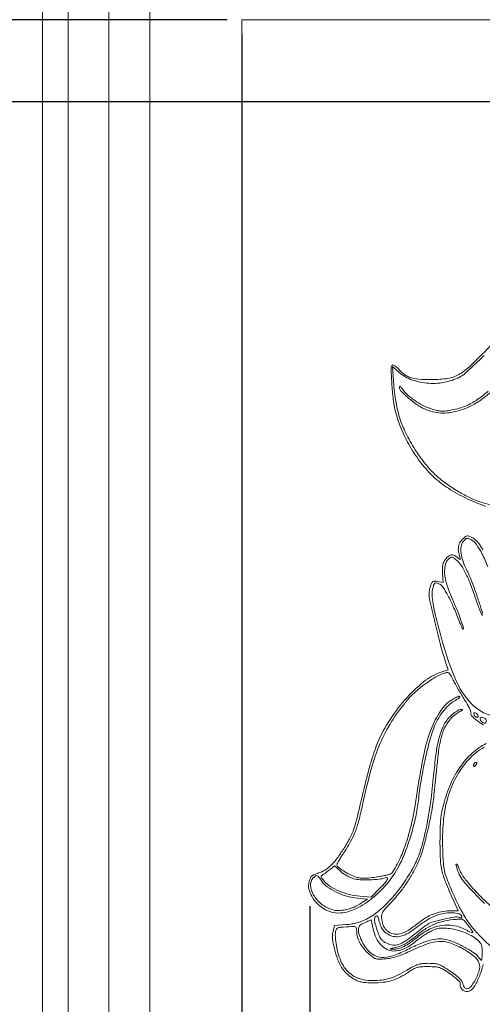
# Model space of a CAD drawing. Units: inches. Extents: x 2656 to 9931, y 1941 to 3068.
# Tile 32 of 46: x 2817 to 2837, y 2952 to 2994. Entities that reach past the tile are written whole.
import ezdxf

# ---------------------------------------------------------------- set-up
doc = ezdxf.new("R2010")
doc.units = ezdxf.units.IN
for name, color, linetype, lineweight in [('A-ANNO-DIMS', 2, 'Continuous', 18), ('A-ELEV-FNSH', 8, 'Continuous', 13), ('A-ELEV-ORN', 8, 'Continuous', 13)]:
    doc.layers.add(name, color=color, linetype=linetype, lineweight=lineweight)
doc.styles.get("Standard").update_dxf_attribs({"font": 'arial.ttf'})
doc.dimstyles.new('ISO-25', dxfattribs={"dimtxt": 6, "dimasz": 2.5, "dimexe": 1.25, "dimexo": 0.625, "dimtad": 1, "dimdec": 0, "dimlunit": 3, "dimtxsty": 'Standard', "dimcen": 2.5, "dimadec": 0, "dimazin": 0, "dimtfac": 1, "dimtdec": 0, "dimtmove": 0, "dimatfit": 3, "dimfxl": 1, "dimarcsym": 0})

# ---------------------------------------------------------------- blocks, each defined once
blk = doc.blocks.new('*D151')
at = {"layer": 'A-ANNO-DIMS', "color": 0, "lineweight": -2, "transparency": 16777216}
for p, q in [((2829.546, 2956.424), (2829.546, 2703.709)), ((2867.059, 2955.98), (2867.059, 2703.709)), ((2832.046, 2704.959), (2864.559, 2704.959))]:
    blk.add_line(p, q, dxfattribs=at)
at = {"layer": 'A-ANNO-DIMS', "color": 0, "transparency": 16777216}
for points in [[(2832.046, 2705.376), (2832.046, 2704.543), (2829.546, 2704.959)], [(2864.559, 2705.376), (2864.559, 2704.543), (2867.059, 2704.959)]]:
    blk.add_solid(points, dxfattribs=at)
at = {"layer": 'Defpoints', "color": 0, "transparency": 16777216}
for p in [(2829.546, 2957.049), (2867.059, 2956.605), (2867.059, 2704.959)]:
    blk.add_point(p, dxfattribs=at)
at = {"layer": 'A-ANNO-DIMS', "color": 0, "transparency": 16777216, "insert": (2848.302, 2708.689), "char_height": 6, "attachment_point": 5}
blk.add_mtext('3\'-1 1/2"', dxfattribs=at)
blk = doc.blocks.new('*D152')
at = {"layer": 'A-ANNO-DIMS', "color": 0, "lineweight": -2, "transparency": 16777216}
for p, q in [((2847.28, 2990.828), (2707.323, 2990.828)), ((2708.573, 2988.328), (2708.573, 2952.971)), ((2847.248, 2950.471), (2707.323, 2950.471))]:
    blk.add_line(p, q, dxfattribs=at)
at = {"layer": 'A-ANNO-DIMS', "color": 0, "transparency": 16777216}
for points in [[(2708.156, 2988.328), (2708.989, 2988.328), (2708.573, 2990.828)], [(2708.156, 2952.971), (2708.989, 2952.971), (2708.573, 2950.471)]]:
    blk.add_solid(points, dxfattribs=at)
at = {"layer": 'Defpoints', "color": 0, "transparency": 16777216}
for p in [(2847.905, 2990.828), (2708.573, 2950.471), (2847.873, 2950.471)]:
    blk.add_point(p, dxfattribs=at)
at = {"layer": 'A-ANNO-DIMS', "color": 0, "transparency": 16777216, "insert": (2704.843, 2970.649), "char_height": 6, "attachment_point": 5, "rotation": 90}
blk.add_mtext('3\'-4 1/2"', dxfattribs=at)
blk = doc.blocks.new('*D153')
at = {"layer": 'A-ANNO-DIMS', "color": 0, "lineweight": -2, "transparency": 16777216}
for p, q in [((2826.64, 2993.722), (2826.64, 2703.709)), ((2829.546, 2956.424), (2829.546, 2703.709)), ((2824.14, 2704.959), (2821.64, 2704.959)), ((2826.64, 2704.959), (2829.546, 2704.959)), ((2832.046, 2704.959), (2851.745, 2704.959))]:
    blk.add_line(p, q, dxfattribs=at)
at = {"layer": 'A-ANNO-DIMS', "color": 0, "transparency": 16777216}
for points in [[(2824.14, 2705.376), (2824.14, 2704.543), (2826.64, 2704.959)], [(2832.046, 2705.376), (2832.046, 2704.543), (2829.546, 2704.959)]]:
    blk.add_solid(points, dxfattribs=at)
at = {"layer": 'Defpoints', "color": 0, "transparency": 16777216}
for p in [(2826.64, 2994.347), (2829.546, 2957.049), (2829.546, 2704.959)]:
    blk.add_point(p, dxfattribs=at)
at = {"layer": 'A-ANNO-DIMS', "color": 0, "transparency": 16777216, "insert": (2843.145, 2708.65), "char_height": 6, "attachment_point": 5}
blk.add_mtext('0\'-3"', dxfattribs=at)
blk = doc.blocks.new('*D154')
at = {"layer": 'A-ANNO-DIMS', "color": 0, "lineweight": -2, "transparency": 16777216}
for p, q in [((2708.573, 2996.847), (2708.573, 2999.347)), ((2826.015, 2994.347), (2707.323, 2994.347)), ((2708.573, 2994.347), (2708.573, 2990.828)), ((2847.28, 2990.828), (2707.323, 2990.828)), ((2708.573, 2988.328), (2708.573, 2954.647))]:
    blk.add_line(p, q, dxfattribs=at)
at = {"layer": 'A-ANNO-DIMS', "color": 0, "transparency": 16777216}
for points in [[(2708.156, 2996.847), (2708.989, 2996.847), (2708.573, 2994.347)], [(2708.156, 2988.328), (2708.989, 2988.328), (2708.573, 2990.828)]]:
    blk.add_solid(points, dxfattribs=at)
at = {"layer": 'Defpoints', "color": 0, "transparency": 16777216}
for p in [(2826.64, 2994.347), (2708.573, 2990.828), (2847.905, 2990.828)]:
    blk.add_point(p, dxfattribs=at)
at = {"layer": 'A-ANNO-DIMS', "color": 0, "transparency": 16777216, "insert": (2704.843, 2970.237), "char_height": 6, "attachment_point": 5, "rotation": 90}
blk.add_mtext('0\'-3 1/2"', dxfattribs=at)

msp = doc.modelspace()

# ---------------------------------------------------------------- linework, layer by layer
at = {"layer": 'A-ELEV-FNSH'}
for p, q in [((2818.129, 2887.893), (2818.129, 2998.286)), ((2819.227, 2887.893), (2819.227, 2998.286)), ((2820.954, 2887.893), (2820.954, 2998.286)), ((2822.705, 2887.893), (2822.705, 2998.286))]:
    msp.add_line(p, q, dxfattribs=at)
msp.add_lwpolyline([(2826.64, 2994.347), (2868.226, 2994.347), (2868.226, 2892.035), (2826.64, 2892.035)], close=True, dxfattribs=at)
at = {"layer": 'A-ELEV-ORN'}
for points in [[(2837.388, 2980.515, -0.006917), (2836.411, 2979.542, -0.058589), (2835.919, 2979.166, -0.098552), (2835.454, 2979.002, -0.035601), (2834.753, 2978.952, -0.016594), (2834.198, 2978.971, -0.061567), (2833.854, 2979.037, -0.083701), (2833.594, 2979.172, -0.049195), (2833.335, 2979.41, 0.027869), (2833.259, 2979.486, 0.040712), (2833.184, 2979.543, 0.047221), (2833.12, 2979.576, 0.237732), (2833.081, 2979.573, 0.271003), (2833.022, 2979.463, 0.005074), (2833.057, 2978.784, 0.012637), (2833.115, 2978.118, 0.031418), (2833.2, 2977.637, 0.038435), (2833.453, 2976.86, 0.033423), (2833.832, 2976.093, 0.033468), (2834.309, 2975.384, 0.038851), (2834.855, 2974.781, 0.047803), (2835.471, 2974.302, 0.029742), (2836.272, 2973.858, 0.029582), (2837.076, 2973.53, 0.082237)], [(2837.268, 2973.607, -0.036465), (2836.854, 2973.712, -0.031934), (2836.41, 2973.892, -0.020481), (2835.919, 2974.154, -0.022981), (2835.355, 2974.522, -0.033565), (2834.898, 2974.9, -0.033845), (2834.498, 2975.333, -0.023918), (2834.107, 2975.868, -0.027291), (2833.693, 2976.58, -0.039588), (2833.413, 2977.251, -0.037719), (2833.235, 2977.982, -0.021941), (2833.126, 2978.88), (2833.078, 2979.51), (2833.373, 2979.257, 0.093666), (2833.935, 2978.935, 0.069007), (2834.64, 2978.795, 0.067281), (2835.375, 2978.85, 0.079378), (2836.025, 2979.101, 0.051813), (2836.194, 2979.224, 0.005013), (2836.567, 2979.568, 0.006325), (2837.004, 2979.988, 0.004959)], [(2837.173, 2978.463, -0.04137), (2836.639, 2978.049, -0.055454), (2836.14, 2977.797, -0.045449), (2835.563, 2977.64, -0.018148), (2835.319, 2977.606, -0.046687), (2835.142, 2977.605, -0.044718), (2834.963, 2977.636, -0.015523), (2834.712, 2977.713, -0.036325), (2834.365, 2977.859, -0.033508), (2834.032, 2978.057, -0.034848), (2833.744, 2978.287, -0.052266), (2833.532, 2978.529, 0.02097), (2833.474, 2978.603, 0.058684), (2833.426, 2978.648, 0.191986), (2833.397, 2978.656, 0.378361), (2833.382, 2978.639, 0.197397), (2833.458, 2978.453, 0.021796), (2833.803, 2978.134, 0.027297), (2834.197, 2977.834, 0.059288), (2834.534, 2977.66, 0.037365), (2834.896, 2977.555, 0.050304), (2835.236, 2977.518, 0.047743), (2835.589, 2977.549, 0.029434), (2835.995, 2977.649, 0.043097), (2836.475, 2977.845, 0.04115), (2836.923, 2978.123, 0.031024), (2837.416, 2978.538, 0.011839)], [(2836.947, 2971.671), (2836.821, 2971.88, 0.042011), (2836.756, 2971.968, 0.026179), (2836.668, 2972.059, 0.026193), (2836.57, 2972.141, 0.042471), (2836.479, 2972.199, 0.021647), (2836.344, 2972.262, 0.13905), (2836.269, 2972.27, 0.136219), (2836.201, 2972.239, 0.020472), (2836.089, 2972.135, 0.032677), (2835.995, 2972.028, 0.065311), (2835.939, 2971.931, 0.063788), (2835.908, 2971.82, 0.029875), (2835.897, 2971.673, 0.050625), (2835.899, 2971.65, 0.003583), (2835.911, 2971.587, 0.005029), (2835.927, 2971.511, 0.00377), (2835.945, 2971.429, -0.004692), (2835.977, 2971.29, -0.249682), (2835.97, 2971.265, -0.396318), (2835.949, 2971.264, -0.007959), (2835.861, 2971.341, 0.070536), (2835.725, 2971.433, 0.149657), (2835.6, 2971.452, 0.136653), (2835.478, 2971.399, 0.054831), (2835.35, 2971.268, 0.045274), (2835.273, 2971.15, 0.070141), (2835.231, 2971.036, 0.05336), (2835.217, 2970.894, 0.016308), (2835.225, 2970.677), (2835.254, 2970.279), (2835.023, 2970.317, 0.027685), (2834.893, 2970.331, 0.129437), (2834.819, 2970.315, 0.147269), (2834.768, 2970.267, 0.039491), (2834.72, 2970.165, 0.026094), (2834.692, 2970.079, 0.016941), (2834.669, 2969.978, 0.017041), (2834.653, 2969.877, 0.030773), (2834.648, 2969.793, 0.055689), (2834.681, 2969.498, 0.002741), (2834.903, 2968.54, 0.004705), (2835.135, 2967.603, 0.01717), (2835.309, 2967.015), (2835.466, 2966.543), (2835.164, 2966.44, 0.088958), (2834.415, 2966.025, 0.041928), (2833.615, 2965.254, 0.040125), (2832.898, 2964.29, 0.047822), (2832.392, 2963.278, 0.016477), (2832.237, 2962.834, 0.009651), (2832.079, 2962.292, 0.006465), (2831.889, 2961.549, 0.001966), (2831.62, 2960.419, -0.01084), (2831.488, 2959.908, -0.029686), (2831.366, 2959.556, -0.032001), (2831.209, 2959.236, -0.014414), (2830.965, 2958.837, -0.01728), (2830.681, 2958.432, -0.041121), (2830.436, 2958.158, -0.053262), (2830.195, 2957.974, -0.056558), (2829.924, 2957.848, 0.020528), (2829.742, 2957.779, 0.074541), (2829.637, 2957.715, 0.099076), (2829.572, 2957.633, 0.053866), (2829.526, 2957.512, 0.15275), (2829.546, 2957.049, 0.098781), (2829.825, 2956.586, 0.093752), (2830.278, 2956.246, 0.12043), (2830.784, 2956.134, 0.103524), (2831.45, 2956.289, 0.056804), (2832.168, 2956.728, 0.052352), (2832.835, 2957.371, 0.05273), (2833.352, 2958.136, 0.031392), (2833.623, 2958.734, 0.018241), (2833.876, 2959.481, 0.018124), (2834.078, 2960.257, 0.027242), (2834.191, 2960.947, -0.013262), (2834.304, 2961.779, -0.01169), (2834.466, 2962.64, -0.012107), (2834.654, 2963.433, -0.024068), (2834.848, 2964.049, -0.039147), (2835.009, 2964.4, -0.035039), (2835.229, 2964.735, -0.036642), (2835.477, 2965.017, -0.064037), (2835.725, 2965.204, 0.014815), (2835.92, 2965.323, 0.249045), (2835.955, 2965.386, 0.545936), (2835.919, 2965.411, 0.017435), (2835.727, 2965.319, 0.116418), (2835.197, 2964.861, 0.061253), (2834.775, 2964.094, 0.042971), (2834.434, 2962.974, 0.017416), (2834.156, 2961.401, -0.008299), (2834.041, 2960.668, -0.012804), (2833.914, 2960.04, -0.014133), (2833.767, 2959.468, -0.014418), (2833.588, 2958.909, -0.020809), (2833.455, 2958.575, -0.016344), (2833.284, 2958.225, -0.01312), (2833.112, 2957.92, -0.108105), (2833.003, 2957.805, -0.094011), (2832.952, 2957.782, -0.005458), (2832.786, 2957.746, -0.008132), (2832.586, 2957.708, -0.005882), (2832.361, 2957.672, -0.009722), (2832.06, 2957.633, -0.027864), (2831.849, 2957.622, -0.037878), (2831.679, 2957.635, -0.038164), (2831.513, 2957.674, -0.039764), (2831.257, 2957.778, -0.027675), (2830.987, 2957.933, -0.021679), (2830.758, 2958.097, -0.230931), (2830.709, 2958.196, -0.124312), (2830.722, 2958.247, -0.00671), (2830.802, 2958.391, -0.010138), (2830.905, 2958.561, -0.007198), (2831.026, 2958.748, 0.023092), (2831.295, 2959.192, 0.032749), (2831.489, 2959.612, 0.028048), (2831.646, 2960.099, 0.011933), (2831.804, 2960.767, -0.015056), (2832.171, 2962.284, -0.033781), (2832.561, 2963.402, -0.040276), (2833.048, 2964.33, -0.032755), (2833.71, 2965.237, -0.038197), (2834.032, 2965.569, -0.02193), (2834.466, 2965.919, -0.021763), (2834.912, 2966.219, -0.055703), (2835.264, 2966.384, -0.035274), (2835.411, 2966.422, -0.201072), (2835.488, 2966.405, -0.115665), (2835.553, 2966.333, -0.00859), (2835.678, 2966.095, 0.010547), (2835.77, 2965.922, 0.004757), (2835.897, 2965.698, 0.004707), (2836.037, 2965.464, 0.006406), (2836.167, 2965.256, -0.013223), (2836.282, 2965.067, -0.018761), (2836.373, 2964.894, -0.015074), (2836.437, 2964.748, -0.18991), (2836.437, 2964.689, 0.295249), (2836.461, 2964.576, 0.02979), (2836.676, 2964.385, 0.030498), (2836.978, 2964.174, 0.021207)], [(2836.938, 2968.965, -0.007722), (2836.907, 2969.052, -0.000935), (2836.843, 2969.243, -0.001111), (2836.768, 2969.472, -0.000915), (2836.689, 2969.716, 0.009573), (2836.598, 2969.981, 0.006843), (2836.487, 2970.275, 0.006912), (2836.373, 2970.551, 0.014682), (2836.275, 2970.762, -0.029108), (2836.098, 2971.176, -0.055084), (2836.012, 2971.528, -0.073018), (2836.018, 2971.814, -0.131428), (2836.114, 2972.026, -0.022465), (2836.205, 2972.128, -0.150284), (2836.265, 2972.16, -0.152301), (2836.331, 2972.153, -0.023261), (2836.453, 2972.093, -0.115515), (2836.671, 2971.897, -0.033174), (2836.908, 2971.506, -0.025971), (2837.163, 2970.944, -0.011782)], [(2837.333, 2964.57, -0.140752), (2836.461, 2965.084, -0.092959), (2835.747, 2966.191, -0.032658), (2835.146, 2967.993, -0.003626), (2834.925, 2968.861, -0.016522), (2834.817, 2969.371, -0.028491), (2834.776, 2969.714, -0.067072), (2834.794, 2969.971, -0.020228), (2834.843, 2970.166, -0.163087), (2834.895, 2970.24, -0.240059), (2834.97, 2970.253, -0.046671), (2835.101, 2970.198, -0.128167), (2835.25, 2970.06, -0.019908), (2835.454, 2969.712, -0.019363), (2835.681, 2969.243, -0.011229), (2835.919, 2968.664, 0.007901), (2835.985, 2968.499, 0.01544), (2836.045, 2968.37, 0.015009), (2836.092, 2968.281, 0.647661), (2836.109, 2968.282, 0.166095), (2836.108, 2968.371, 0.003358), (2835.956, 2968.796, 0.008477), (2835.783, 2969.246, 0.009943), (2835.603, 2969.666, -0.031396), (2835.4, 2970.205, -0.056644), (2835.313, 2970.669, -0.075376), (2835.342, 2971.035, -0.152708), (2835.487, 2971.282, -0.047306), (2835.568, 2971.342, -0.186308), (2835.628, 2971.353, -0.114576), (2835.697, 2971.322, -0.013223), (2835.831, 2971.215, -0.070968), (2836.022, 2971.002, -0.031699), (2836.211, 2970.676, -0.024153), (2836.407, 2970.227, -0.010905), (2836.624, 2969.621, 0.006458), (2836.712, 2969.364, 0.008923), (2836.799, 2969.137, 0.006081), (2836.877, 2968.95, 0.101504), (2836.916, 2968.895, 0.046443), (2836.947, 2968.87, 0.495533)], [(2837.09, 2963.393, 0.063336), (2836.491, 2962.974, 0.055528), (2835.985, 2962.402, 0.050333), (2835.577, 2961.677, 0.03685), (2835.271, 2960.806, 0.019452), (2835.194, 2960.471, 0.022521), (2835.147, 2960.146, 0.017152), (2835.123, 2959.754, 0.005963), (2835.114, 2959.188, 0.012907), (2835.13, 2958.437, 0.04431), (2835.196, 2957.954, 0.040715), (2835.349, 2957.469, 0.009684), (2835.684, 2956.692), (2835.891, 2956.234), (2835.523, 2956.229, 0.045199), (2835.169, 2956.192, 0.044452), (2834.826, 2956.091, 0.042871), (2834.494, 2955.928, 0.036571), (2834.176, 2955.702, -0.030516), (2833.749, 2955.391, -0.081318), (2833.404, 2955.243, -0.119643), (2833.113, 2955.241, -0.120092), (2832.854, 2955.373, -0.051291), (2832.77, 2955.462, -0.050194), (2832.705, 2955.566, -0.046486), (2832.659, 2955.689, -0.033937), (2832.63, 2955.832, -0.039809), (2832.619, 2956.023, -0.11251), (2832.652, 2956.151, -0.065107), (2832.748, 2956.29, -0.007365), (2833.008, 2956.57, 0.019968), (2833.322, 2956.925, 0.019223), (2833.61, 2957.308, 0.018549), (2833.877, 2957.725, 0.015887), (2834.128, 2958.183, 0.045112), (2834.332, 2958.695, 0.012919), (2834.554, 2959.521, 0.01347), (2834.744, 2960.415, 0.021086), (2834.855, 2961.193, -0.002506), (2835.023, 2962.803, -0.022088), (2835.132, 2963.51, -0.050263), (2835.266, 2963.95, -0.057275), (2835.482, 2964.333, -0.030263), (2835.577, 2964.449, -0.022363), (2835.695, 2964.565, -0.022756), (2835.817, 2964.665, -0.046205), (2835.922, 2964.73, 0.015427), (2836.008, 2964.775, 0.045541), (2836.062, 2964.813, 0.188236), (2836.074, 2964.836, 0.446394), (2836.063, 2964.849, 0.130235), (2835.898, 2964.808, 0.042316), (2835.687, 2964.668, 0.041107), (2835.482, 2964.475, 0.051459), (2835.327, 2964.265, 0.049393), (2835.157, 2963.894, 0.031219), (2835.029, 2963.435, 0.021609), (2834.926, 2962.811, 0.007321), (2834.828, 2961.896, -0.012313), (2834.69, 2960.722, -0.017737), (2834.506, 2959.693, -0.020279), (2834.285, 2958.837, -0.043505), (2834.032, 2958.204, -0.032081), (2833.6, 2957.47, -0.032116), (2833.079, 2956.798, -0.034114), (2832.519, 2956.246, -0.057459), (2831.973, 2955.876, -0.024989), (2831.768, 2955.781, -0.02907), (2831.564, 2955.713, -0.027774), (2831.345, 2955.667, -0.019652), (2831.096, 2955.638), (2830.604, 2955.601), (2830.541, 2955.345, 0.04489), (2830.518, 2955.199, 0.035063), (2830.519, 2955.038, 0.0281), (2830.545, 2954.847, 0.013749), (2830.598, 2954.607, 0.028366), (2830.737, 2954.159, 0.049961), (2830.908, 2953.812, 0.058686), (2831.122, 2953.545, 0.062175), (2831.388, 2953.341, 0.027979), (2831.58, 2953.242, 0.049342), (2831.75, 2953.186, 0.040392), (2831.949, 2953.158, 0.01307), (2832.247, 2953.148, 0.030789), (2832.683, 2953.171, 0.045035), (2833.059, 2953.25, 0.045895), (2833.409, 2953.393, 0.033673), (2833.768, 2953.611, -0.022313), (2833.971, 2953.741, -0.063467), (2834.125, 2953.806, -0.054529), (2834.303, 2953.835, -0.01333), (2834.601, 2953.843, -0.014709), (2834.915, 2953.834, -0.064568), (2835.096, 2953.799, -0.06152), (2835.267, 2953.719, -0.012586), (2835.545, 2953.533, -0.011868), (2835.713, 2953.409, -0.01771), (2835.854, 2953.292, -0.012896), (2835.961, 2953.19, -0.229837), (2835.977, 2953.147, 0.109568), (2835.994, 2952.981, 0.12714), (2836.08, 2952.848, 0.138612), (2836.213, 2952.781, 0.140792), (2836.36, 2952.793, 0.168464), (2836.572, 2952.972, 0.037603), (2836.785, 2953.4, 0.03671), (2836.959, 2953.937, 0.036373)], [(2837.709, 2954.391, -0.040006), (2836.914, 2955.06, -0.026392), (2836.523, 2955.489, -0.0308), (2836.201, 2955.936, -0.026889), (2835.904, 2956.468, -0.013877), (2835.588, 2957.162, -0.00869), (2835.391, 2957.651, -0.039149), (2835.304, 2957.946, -0.035615), (2835.26, 2958.263, -0.006374), (2835.228, 2958.86, -0.032346), (2835.257, 2960.049, -0.047785), (2835.448, 2961.073, -0.053817), (2835.804, 2961.946, -0.061487), (2836.326, 2962.681, -0.03606), (2836.648, 2962.986, -0.039542), (2837.002, 2963.232, -0.037445)], [(2837.365, 2956.361, -0.021757), (2836.712, 2956.983, -0.023987), (2836.211, 2957.554, -0.067202), (2835.939, 2958.01, 0.007616), (2835.855, 2958.2, 0.23927), (2835.816, 2958.231, 0.54885), (2835.795, 2958.21, 0.010042), (2835.843, 2958.03, 0.110716), (2836.169, 2957.433, 0.021714), (2837.019, 2956.546, 0.024103)]]:
    msp.add_lwpolyline(points, format="xyb", dxfattribs=at)
for points in [[(2836.745, 2964.573, -0.08306), (2836.75, 2964.539, -0.196386), (2836.74, 2964.516, -0.196386), (2836.717, 2964.506, -0.08306), (2836.683, 2964.512, -0.068635), (2836.646, 2964.53, -0.04742), (2836.609, 2964.561, -0.04742), (2836.579, 2964.597, -0.068635), (2836.56, 2964.635, -0.08306), (2836.555, 2964.669, -0.196386), (2836.565, 2964.692, -0.196386), (2836.588, 2964.702, -0.08306), (2836.622, 2964.696, -0.068635), (2836.659, 2964.678, -0.04742), (2836.696, 2964.648, -0.04742), (2836.726, 2964.611, -0.068635)], [(2837.075, 2964.428, -0.133358), (2837.099, 2964.346, -0.215554), (2837.071, 2964.28, -0.223994), (2837.004, 2964.259, -0.139938), (2836.928, 2964.293, -0.033484), (2836.89, 2964.329, -0.035275), (2836.858, 2964.369, -0.037707), (2836.835, 2964.408, -0.113581), (2836.828, 2964.437, -0.291763), (2836.857, 2964.482, -0.118104), (2836.931, 2964.497, -0.094142), (2837.018, 2964.477, -0.152872)], [(2836.594, 2962.553, 0.063896), (2836.576, 2962.529, 0.039129), (2836.561, 2962.498, 0.038674), (2836.55, 2962.464, 0.054831), (2836.547, 2962.433, 0.142677), (2836.554, 2962.411, 0.290264), (2836.57, 2962.403, 0.131573), (2836.596, 2962.414, 0.034019), (2836.63, 2962.444, 0.041736), (2836.659, 2962.478, 0.061283), (2836.678, 2962.513, 0.080535), (2836.685, 2962.543, 0.212536), (2836.677, 2962.563, 0.128169), (2836.66, 2962.574, 0.100736), (2836.638, 2962.575, 0.089268), (2836.615, 2962.568, 0.075941)], [(2831.426, 2957.602, 0.055433), (2831.704, 2957.558, 0.01871), (2832.113, 2957.556, 0.018199), (2832.518, 2957.583, 0.066652), (2832.767, 2957.643, -0.208313), (2832.85, 2957.64, -0.418459), (2832.869, 2957.584, -0.064234), (2832.764, 2957.428, -0.012489), (2832.533, 2957.179), (2832.176, 2956.813), (2831.689, 2956.853, -0.041654), (2831.248, 2956.928, -0.036916), (2830.806, 2957.076, -0.038773), (2830.424, 2957.273, -0.079799), (2830.17, 2957.492, -0.010258), (2830.063, 2957.625, -0.116062), (2830.035, 2957.686, -0.252336), (2830.049, 2957.731, -0.06286), (2830.113, 2957.78, 0.018651), (2830.173, 2957.818, 0.007118), (2830.254, 2957.875, 0.007037), (2830.341, 2957.94, 0.00857), (2830.42, 2958.003), (2830.602, 2958.155), (2830.863, 2957.919, 0.033265), (2830.984, 2957.823, 0.02209), (2831.136, 2957.729, 0.022262), (2831.291, 2957.65, 0.039835)], [(2830.063, 2957.494, 0.096696), (2830.293, 2957.255, 0.04079), (2830.679, 2957.03, 0.039179), (2831.134, 2956.854, 0.047452), (2831.582, 2956.765), (2832.01, 2956.722), (2831.764, 2956.565, -0.041448), (2831.44, 2956.393, -0.043479), (2831.098, 2956.281, -0.047273), (2830.776, 2956.238, -0.087815), (2830.515, 2956.273, -0.08927), (2830.054, 2956.518, -0.090925), (2829.711, 2956.906, -0.114994), (2829.578, 2957.317, -0.220837), (2829.694, 2957.636, -0.046587), (2829.797, 2957.721, -0.246709), (2829.867, 2957.729, -0.143928), (2829.939, 2957.675, -0.013937)], [(2832.26, 2955.444, 0.062168), (2832.386, 2955.076, 0.075154), (2832.592, 2954.776, 0.085533), (2832.852, 2954.58, 0.119666), (2833.134, 2954.511, 0.055537), (2833.367, 2954.537, 0.048546), (2833.6, 2954.614, 0.043338), (2833.837, 2954.744, 0.02961), (2834.082, 2954.93, -0.019295), (2834.199, 2955.022, -0.00962), (2834.354, 2955.131, -0.009534), (2834.52, 2955.238, -0.013848), (2834.67, 2955.325, -0.021165), (2834.875, 2955.426, -0.055472), (2835.031, 2955.475, -0.052361), (2835.199, 2955.489, -0.01724), (2835.448, 2955.477, -0.036743), (2835.791, 2955.421, -0.034428), (2836.13, 2955.316, -0.035125), (2836.445, 2955.167, -0.042887), (2836.714, 2954.985, -0.066426), (2836.833, 2954.858, -0.09513), (2836.897, 2954.719, -0.062864), (2836.92, 2954.525, -0.01545), (2836.908, 2954.203, -0.04028), (2836.898, 2954.135, -0.434657), (2836.876, 2954.123, -0.144233), (2836.842, 2954.146, -0.007908), (2836.758, 2954.249, 0.081468), (2836.54, 2954.449, 0.021937), (2836.134, 2954.69, 0.022976), (2835.696, 2954.899, 0.05307), (2835.347, 2955.004, 0.060044), (2835.029, 2955.026, 0.0519), (2834.699, 2954.974, 0.036545), (2834.294, 2954.834, 0.012427), (2833.729, 2954.574, -0.024635), (2833.138, 2954.32, -0.076981), (2832.715, 2954.232, -0.113115), (2832.381, 2954.292, -0.095141), (2832.082, 2954.492, -0.050468), (2831.916, 2954.693, -0.0336), (2831.767, 2954.952, -0.033989), (2831.66, 2955.215, -0.078158), (2831.626, 2955.425, -0.077194), (2831.639, 2955.517, -0.107915), (2831.68, 2955.589, -0.079481), (2831.757, 2955.652, -0.026565), (2831.888, 2955.718, 0.000354), (2831.99, 2955.763, 0.000548), (2832.077, 2955.802, 0.000157), (2832.154, 2955.836, 0.018033), (2832.164, 2955.841, -0.489273), (2832.17, 2955.838, -0.001166), (2832.197, 2955.727, -0.005275), (2832.227, 2955.598, -0.003118)], [(2836.041, 2955.995, -0.101928), (2836.045, 2955.957, -0.279733), (2836.03, 2955.936, -0.146843), (2835.993, 2955.932, -0.029839), (2835.929, 2955.948, 0.118654), (2835.728, 2955.962, 0.01344), (2835.276, 2955.875, 0.016099), (2834.829, 2955.76, 0.069263), (2834.578, 2955.648, 0.018343), (2834.485, 2955.584, 0.004448), (2834.335, 2955.472, 0.004556), (2834.166, 2955.341, 0.004517), (2833.998, 2955.206, -0.023572), (2833.625, 2954.928, -0.07208), (2833.341, 2954.791, -0.103356), (2833.092, 2954.766, -0.087157), (2832.836, 2954.84, -0.043102), (2832.689, 2954.928, -0.081644), (2832.592, 2955.026, -0.059486), (2832.514, 2955.17, -0.014373), (2832.42, 2955.425, -0.010192), (2832.348, 2955.657, -0.038677), (2832.317, 2955.806, -0.066595), (2832.317, 2955.908, -0.13947), (2832.349, 2955.98, -0.138824), (2832.394, 2956.01, -0.309109), (2832.432, 2956, -0.092788), (2832.468, 2955.935, -0.011506), (2832.517, 2955.779, 0.027606), (2832.601, 2955.54, 0.070656), (2832.695, 2955.382, 0.080627), (2832.82, 2955.268, 0.044698), (2833.003, 2955.171, 0.093711), (2833.237, 2955.122, 0.079389), (2833.487, 2955.156, 0.062271), (2833.765, 2955.28, 0.031366), (2834.08, 2955.498, -0.011757), (2834.237, 2955.617, -0.008472), (2834.418, 2955.742, -0.008564), (2834.594, 2955.854, -0.018298), (2834.734, 2955.934, -0.057249), (2835.119, 2956.082, -0.051471), (2835.542, 2956.145, -0.056941), (2835.895, 2956.121, -0.273427)], [(2836.361, 2955.549, -0.006438), (2836.509, 2955.341, -0.415328), (2836.502, 2955.301, -0.270531), (2836.452, 2955.298, -0.004341), (2836.188, 2955.429, 0.074239), (2835.684, 2955.598, 0.083136), (2835.174, 2955.603, 0.077675), (2834.662, 2955.438, 0.055173), (2834.155, 2955.109, -0.017292), (2833.834, 2954.863, -0.03757), (2833.568, 2954.703, -0.049413), (2833.337, 2954.614, -0.076493), (2833.125, 2954.589, -0.005485), (2833.007, 2954.594, -0.641201), (2833.003, 2954.605, -0.142065), (2833.027, 2954.619, -0.002048), (2833.193, 2954.659, 0.026819), (2833.437, 2954.73, 0.043686), (2833.634, 2954.819, 0.035275), (2833.839, 2954.955, 0.011651), (2834.12, 2955.181, -0.033856), (2834.513, 2955.469, -0.045116), (2834.906, 2955.671, -0.045222), (2835.328, 2955.799, -0.034251), (2835.809, 2955.865, -0.017242), (2836.015, 2955.872, -0.130304), (2836.108, 2955.847, -0.097415), (2836.188, 2955.777, -0.007569)], [(2831.553, 2955.348, 0.069778), (2831.587, 2955.11, 0.053354), (2831.685, 2954.867, 0.048265), (2831.846, 2954.627, 0.037842), (2832.062, 2954.4, 0.01904), (2832.244, 2954.247, 0.088877), (2832.365, 2954.184, 0.080452), (2832.506, 2954.164, 0.014003), (2832.775, 2954.176, 0.029064), (2833.009, 2954.207, 0.026601), (2833.245, 2954.265, 0.02299), (2833.502, 2954.357, 0.013221), (2833.804, 2954.489, -0.020096), (2834.57, 2954.813, -0.07641), (2835.077, 2954.92, -0.096363), (2835.529, 2954.858, -0.043396), (2836.079, 2954.615, -0.038883), (2836.566, 2954.295, -0.143385), (2836.78, 2954, -0.164297), (2836.786, 2953.662, -0.055511), (2836.583, 2953.205, -0.043532), (2836.425, 2952.982, -0.165856), (2836.281, 2952.896, -0.289388), (2836.166, 2952.938, -0.109703), (2836.091, 2953.1, 0.089433), (2836.042, 2953.217, 0.05213), (2835.947, 2953.336, 0.035311), (2835.792, 2953.471, 0.012222), (2835.55, 2953.645, 0.010478), (2835.247, 2953.843, 0.052102), (2835.064, 2953.932, 0.065242), (2834.886, 2953.972, 0.022173), (2834.621, 2953.984, 0.022721), (2834.364, 2953.972, 0.054132), (2834.178, 2953.934, 0.045578), (2833.985, 2953.853, 0.012362), (2833.697, 2953.69, -0.020375), (2833.294, 2953.471, -0.04091), (2832.957, 2953.338, -0.044402), (2832.622, 2953.269, -0.028844), (2832.226, 2953.246, -0.047941), (2831.851, 2953.281, -0.062135), (2831.522, 2953.388, -0.066114), (2831.246, 2953.566, -0.065547), (2831.025, 2953.81, -0.054609), (2830.877, 2954.081, -0.029155), (2830.754, 2954.442, -0.028573), (2830.669, 2954.832, -0.038323), (2830.64, 2955.192, -0.054594), (2830.661, 2955.388, -0.22086), (2830.731, 2955.481, -0.102044), (2830.886, 2955.527, -0.007729), (2831.325, 2955.555, -0.023788), (2831.459, 2955.555, -0.174033), (2831.518, 2955.531, -0.183842), (2831.546, 2955.476, -0.027104)]]:
    msp.add_lwpolyline(points, format="xyb", close=True, dxfattribs=at)

# ---------------------------------------------------------------- dimensions: what is measured, and where the dimension line sits
at = {"layer": 'A-ANNO-DIMS'}
for base, p1, p2, picture, middle in [((2708.573, 2990.828), (2826.64, 2994.347), (2847.905, 2990.828), '*D154', (2704.843, 2970.237)), ((2708.573, 2950.471), (2847.905, 2990.828), (2847.873, 2950.471), '*D152', (2704.843, 2970.649))]:
    dim = msp.add_linear_dim(base=base, p1=p1, p2=p2, angle=90, dimstyle='ISO-25', override={"dimdec": 1, "dimlfac": 1, "dimrnd": 0, "dimzin": 1, "dimdsep": 46, "dimlunit": 4, "dimfrac": 2}, dxfattribs=at)
    dim.commit()
    dim.dimension.update_dxf_attribs({"geometry": picture, "text_midpoint": middle})
for base, p1, p2, picture, middle in [((2829.546, 2704.959), (2826.64, 2994.347), (2829.546, 2957.049), '*D153', (2843.145, 2708.65)), ((2867.059, 2704.959), (2829.546, 2957.049), (2867.059, 2956.605), '*D151', (2848.302, 2708.689))]:
    dim = msp.add_linear_dim(base=base, p1=p1, p2=p2, dimstyle='ISO-25', override={"dimdec": 1, "dimlfac": 1, "dimrnd": 0, "dimzin": 1, "dimdsep": 46, "dimlunit": 4, "dimfrac": 2}, dxfattribs=at)
    dim.commit()
    dim.dimension.update_dxf_attribs({"geometry": picture, "text_midpoint": middle})

doc.saveas('drawing.dxf')
